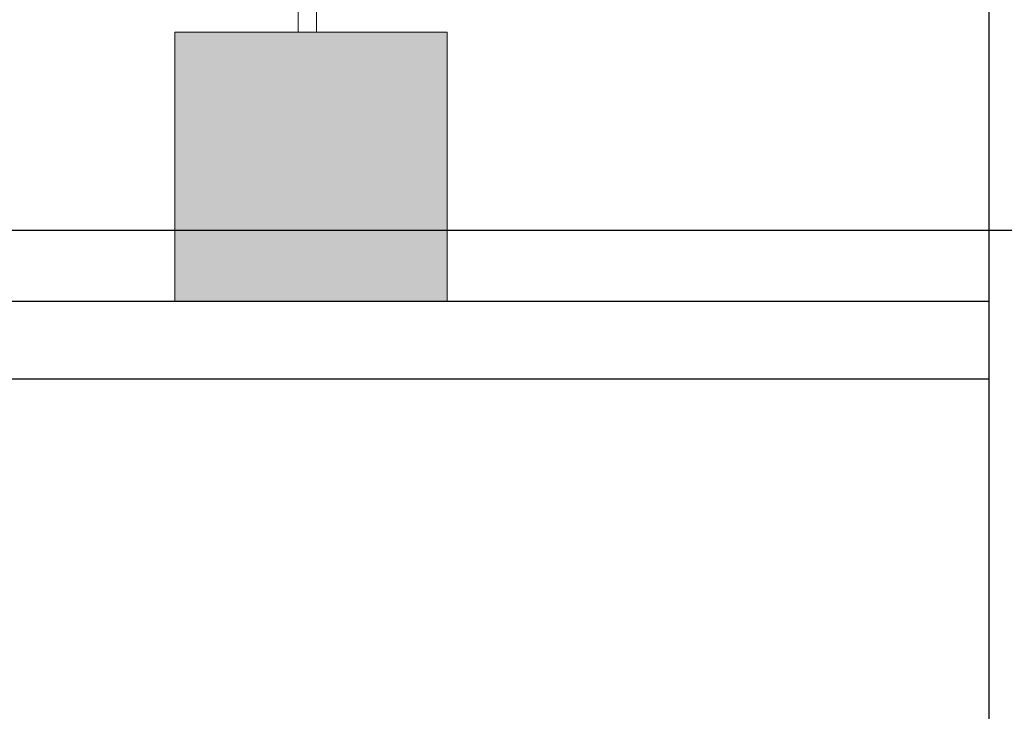
# Model space of a CAD drawing. Units: millimetres. Extents: x 7894 to 8038, y 6851 to 6951.
# Tile 9 of 49: x 7974.616 to 7980.935, y 6870.767 to 6875.21. Entities that reach past the tile are written whole.
import ezdxf

# ---------------------------------------------------------------- set-up
doc = ezdxf.new("R2010")
doc.units = ezdxf.units.MM
for name, color, linetype, lineweight in [('A-ANNO-DIMS', 2, 'Continuous', 18), ('A-FURN-ACCS', 8, 'Continuous', 13), ('A-FURN-SHLF', 7, 'Continuous', 30)]:
    doc.layers.add(name, color=color, linetype=linetype, lineweight=lineweight)
doc.layers.add('A-FURN-ACCS-PATT', color=116, linetype='Continuous', lineweight=9, true_color=0x136734)
doc.styles.get("Standard").update_dxf_attribs({"font": 'arial.ttf'})
doc.dimstyles.new('ISO-25', dxfattribs={"dimtxt": 1, "dimasz": 1, "dimexe": 1.25, "dimexo": 0.625, "dimtad": 1, "dimdec": 0, "dimlunit": 4, "dimtxsty": 'Standard', "dimcen": 2.5, "dimclrt": 1, "dimadec": 0, "dimazin": 0, "dimtfac": 1, "dimtdec": 0, "dimtmove": 0, "dimatfit": 3, "dimfxl": 1, "dimarcsym": 0})

# ---------------------------------------------------------------- blocks, each defined once
blk = doc.blocks.new('*D22')
at = {"layer": 'A-ANNO-DIMS', "color": 0, "lineweight": -2, "transparency": 16777216}
for p, q in [((7983.3131, 6866.2225), (7983.3131, 6876.8981)), ((7981.3426, 6865.2225), (7984.5631, 6865.2225)), ((7983.3131, 6864.7225), (7983.3131, 6865.2225)), ((7981.3426, 6864.7225), (7984.5631, 6864.7225)), ((7983.3131, 6863.7225), (7983.3131, 6862.7225))]:
    blk.add_line(p, q, dxfattribs=at)
at = {"layer": 'A-ANNO-DIMS', "color": 0, "transparency": 16777216}
for points in [[(7983.1464, 6866.2225), (7983.4798, 6866.2225), (7983.3131, 6865.2225)], [(7983.1464, 6863.7225), (7983.4798, 6863.7225), (7983.3131, 6864.7225)]]:
    blk.add_solid(points, dxfattribs=at)
at = {"layer": 'Defpoints', "color": 0, "transparency": 16777216}
for p in [(7980.7176, 6865.2225), (7983.3131, 6865.2225), (7980.7176, 6864.7225)]:
    blk.add_point(p, dxfattribs=at)
at = {"layer": 'A-ANNO-DIMS', "color": 1, "transparency": 16777216, "insert": (7982.171, 6872.0603), "char_height": 1, "attachment_point": 5, "rotation": 90}
blk.add_mtext('0\'-0 1/2" TYP.', dxfattribs=at)
blk = doc.blocks.new('*D36')
at = {"layer": 'A-ANNO-DIMS', "color": 0, "lineweight": -2, "transparency": 16777216}
for p, q in [((7980.8359, 6877.9586), (7980.8359, 6858.5122)), ((7944.4866, 6864.4359), (7944.4866, 6858.5122)), ((7945.4866, 6859.7622), (7979.8359, 6859.7622))]:
    blk.add_line(p, q, dxfattribs=at)
at = {"layer": 'A-ANNO-DIMS', "color": 0, "transparency": 16777216}
for points in [[(7945.4866, 6859.9288), (7945.4866, 6859.5955), (7944.4866, 6859.7622)], [(7979.8359, 6859.9288), (7979.8359, 6859.5955), (7980.8359, 6859.7622)]]:
    blk.add_solid(points, dxfattribs=at)
at = {"layer": 'Defpoints', "color": 0, "transparency": 16777216}
for p in [(7980.8359, 6878.5836), (7944.4866, 6865.0609), (7980.8359, 6859.7622)]:
    blk.add_point(p, dxfattribs=at)
at = {"layer": 'A-ANNO-DIMS', "color": 1, "transparency": 16777216, "insert": (7962.6613, 6860.9046), "char_height": 1, "attachment_point": 5}
blk.add_mtext('3\'-0 1/2"', dxfattribs=at)
blk = doc.blocks.new('*D38')
at = {"layer": 'A-ANNO-DIMS', "color": 0, "lineweight": -2, "transparency": 16777216}
for p, q in [((7981.4609, 6872.9028), (7983.9334, 6872.9028)), ((7982.6834, 6865.7225), (7982.6834, 6871.9028)), ((7981.3426, 6864.7225), (7983.9334, 6864.7225))]:
    blk.add_line(p, q, dxfattribs=at)
at = {"layer": 'A-ANNO-DIMS', "color": 0, "transparency": 16777216}
for points in [[(7982.5168, 6871.9028), (7982.8501, 6871.9028), (7982.6834, 6872.9028)], [(7982.5168, 6865.7225), (7982.8501, 6865.7225), (7982.6834, 6864.7225)]]:
    blk.add_solid(points, dxfattribs=at)
at = {"layer": 'Defpoints', "color": 0, "transparency": 16777216}
for p in [(7980.8359, 6872.9028), (7982.6834, 6872.9028), (7980.7176, 6864.7225)]:
    blk.add_point(p, dxfattribs=at)
at = {"layer": 'A-ANNO-DIMS', "color": 1, "transparency": 16777216, "insert": (7981.5479, 6868.8127), "char_height": 1, "attachment_point": 5, "rotation": 90}
blk.add_mtext('0\'-8"', dxfattribs=at)
blk = doc.blocks.new('*D39')
at = {"layer": 'A-ANNO-DIMS', "color": 0, "lineweight": -2, "transparency": 16777216}
for p, q in [((7982.6834, 6874.8578), (7982.6834, 6879.7661)), ((7964.1574, 6873.8578), (7983.9334, 6873.8578)), ((7982.6834, 6872.9028), (7982.6834, 6873.8578)), ((7981.4609, 6872.9028), (7983.9334, 6872.9028)), ((7982.6834, 6871.9028), (7982.6834, 6870.9028))]:
    blk.add_line(p, q, dxfattribs=at)
at = {"layer": 'A-ANNO-DIMS', "color": 0, "transparency": 16777216}
for points in [[(7982.5168, 6874.8578), (7982.8501, 6874.8578), (7982.6834, 6873.8578)], [(7982.5168, 6871.9028), (7982.8501, 6871.9028), (7982.6834, 6872.9028)]]:
    blk.add_solid(points, dxfattribs=at)
at = {"layer": 'Defpoints', "color": 0, "transparency": 16777216}
for p in [(7963.5324, 6873.8578), (7982.6834, 6873.8578), (7980.8359, 6872.9028)]:
    blk.add_point(p, dxfattribs=at)
at = {"layer": 'A-ANNO-DIMS', "color": 1, "transparency": 16777216, "insert": (7981.5479, 6877.8119), "char_height": 1, "attachment_point": 5, "rotation": 90}
blk.add_mtext('0\'-1"', dxfattribs=at)
blk = doc.blocks.new('*D40')
at = {"layer": 'A-ANNO-DIMS', "color": 0, "lineweight": -2, "transparency": 16777216}
for p, q in [((7982.6834, 6878.5836), (7982.6834, 6885.822)), ((7981.4609, 6878.5836), (7983.9334, 6878.5836)), ((7982.6834, 6874.8578), (7982.6834, 6877.5836)), ((7964.1574, 6873.8578), (7983.9334, 6873.8578))]:
    blk.add_line(p, q, dxfattribs=at)
at = {"layer": 'A-ANNO-DIMS', "color": 0, "transparency": 16777216}
for points in [[(7982.5168, 6877.5836), (7982.8501, 6877.5836), (7982.6834, 6878.5836)], [(7982.5168, 6874.8578), (7982.8501, 6874.8578), (7982.6834, 6873.8578)]]:
    blk.add_solid(points, dxfattribs=at)
at = {"layer": 'Defpoints', "color": 0, "transparency": 16777216}
for p in [(7980.8359, 6878.5836), (7982.6834, 6878.5836), (7963.5324, 6873.8578)]:
    blk.add_point(p, dxfattribs=at)
at = {"layer": 'A-ANNO-DIMS', "color": 1, "transparency": 16777216, "insert": (7981.5414, 6882.7028), "char_height": 1, "attachment_point": 5, "rotation": 90}
blk.add_mtext('0\'-4 1/2"', dxfattribs=at)

msp = doc.modelspace()

# ---------------------------------------------------------------- hatches: boundary and pattern name
at = {"layer": 'A-FURN-ACCS-PATT'}
h = msp.add_hatch(color=256, dxfattribs=at)
h.dxf.hatch_style = 1
h.paths.add_polyline_path([(7977.3595, 6875.13), (7976.5208, 6875.13), (7976.402, 6875.13), (7975.6117, 6875.13), (7975.6117, 6873.4028), (7977.3595, 6873.4028)])

# ---------------------------------------------------------------- linework, layer by layer
at = {"layer": 'A-FURN-ACCS'}
for p, q in [((7976.402, 6875.13, 2.197), (7976.402, 6876.1672, 2.197)), ((7976.5208, 6875.13, 2.197), (7976.5208, 6876.1224, 2.197)), ((7975.6117, 6873.4028, 2.197), (7975.6117, 6875.13, 2.197)), ((7975.6117, 6875.13, 2.197), (7976.402, 6875.13, 2.197)), ((7976.5208, 6875.13, 2.197), (7976.402, 6875.13, 2.197)), ((7976.5208, 6875.13, 2.197), (7977.3595, 6875.13, 2.197)), ((7977.3595, 6873.4028, 2.197), (7977.3595, 6875.13, 2.197))]:
    msp.add_line(p, q, dxfattribs=at)
at = {"layer": 'A-FURN-SHLF'}
for p, q in [((7963.5324, 6873.4028, 2.197), (7980.8359, 6873.4028, 2.197)), ((7980.8359, 6873.4028, 2.197), (7980.8359, 6872.9028, 2.197)), ((7963.5324, 6872.9028, 2.197), (7980.8359, 6872.9028, 2.197))]:
    msp.add_line(p, q, dxfattribs=at)

# ---------------------------------------------------------------- dimensions: what is measured, and where the dimension line sits
at = {"layer": 'A-ANNO-DIMS'}
for base, p1, p2, picture, middle in [((7982.6834, 6878.5836), (7963.5324, 6873.8578), (7980.8359, 6878.5836), '*D40', (7981.5414, 6882.7028)), ((7982.6834, 6873.8578), (7980.8359, 6872.9028), (7963.5324, 6873.8578), '*D39', (7981.5479, 6877.8119)), ((7982.6834, 6872.9028), (7980.7176, 6864.7225), (7980.8359, 6872.9028), '*D38', (7981.5479, 6868.8127))]:
    dim = msp.add_linear_dim(base=base, p1=p1, p2=p2, angle=90, dimstyle='ISO-25', override={"dimdec": 1, "dimlfac": 1, "dimrnd": 0, "dimzin": 1, "dimdsep": 46, "dimlunit": 4, "dimfrac": 2}, dxfattribs=at)
    dim.commit()
    dim.dimension.update_dxf_attribs({"geometry": picture, "text_midpoint": middle})
dim = msp.add_linear_dim(base=(7980.8359, 6859.7622), p1=(7944.4866, 6865.0609), p2=(7980.8359, 6878.5836), dimstyle='ISO-25', override={"dimdec": 1, "dimlfac": 1, "dimrnd": 0, "dimzin": 1, "dimdsep": 46, "dimlunit": 4, "dimfrac": 2}, dxfattribs=at)
dim.commit()
dim.dimension.update_dxf_attribs({"geometry": '*D36', "text_midpoint": (7962.6613, 6860.9046)})
dim = msp.add_linear_dim(base=(7983.3131, 6865.2225), p1=(7980.7176, 6864.7225), p2=(7980.7176, 6865.2225), angle=90, text='<> TYP.', dimstyle='ISO-25', override={"dimdec": 1, "dimlfac": 1, "dimrnd": 0, "dimzin": 1, "dimdsep": 46, "dimlunit": 4, "dimfrac": 2}, dxfattribs=at)
dim.commit()
dim.dimension.update_dxf_attribs({"geometry": '*D22', "text_midpoint": (7982.171, 6872.0603)})

doc.saveas('drawing.dxf')
